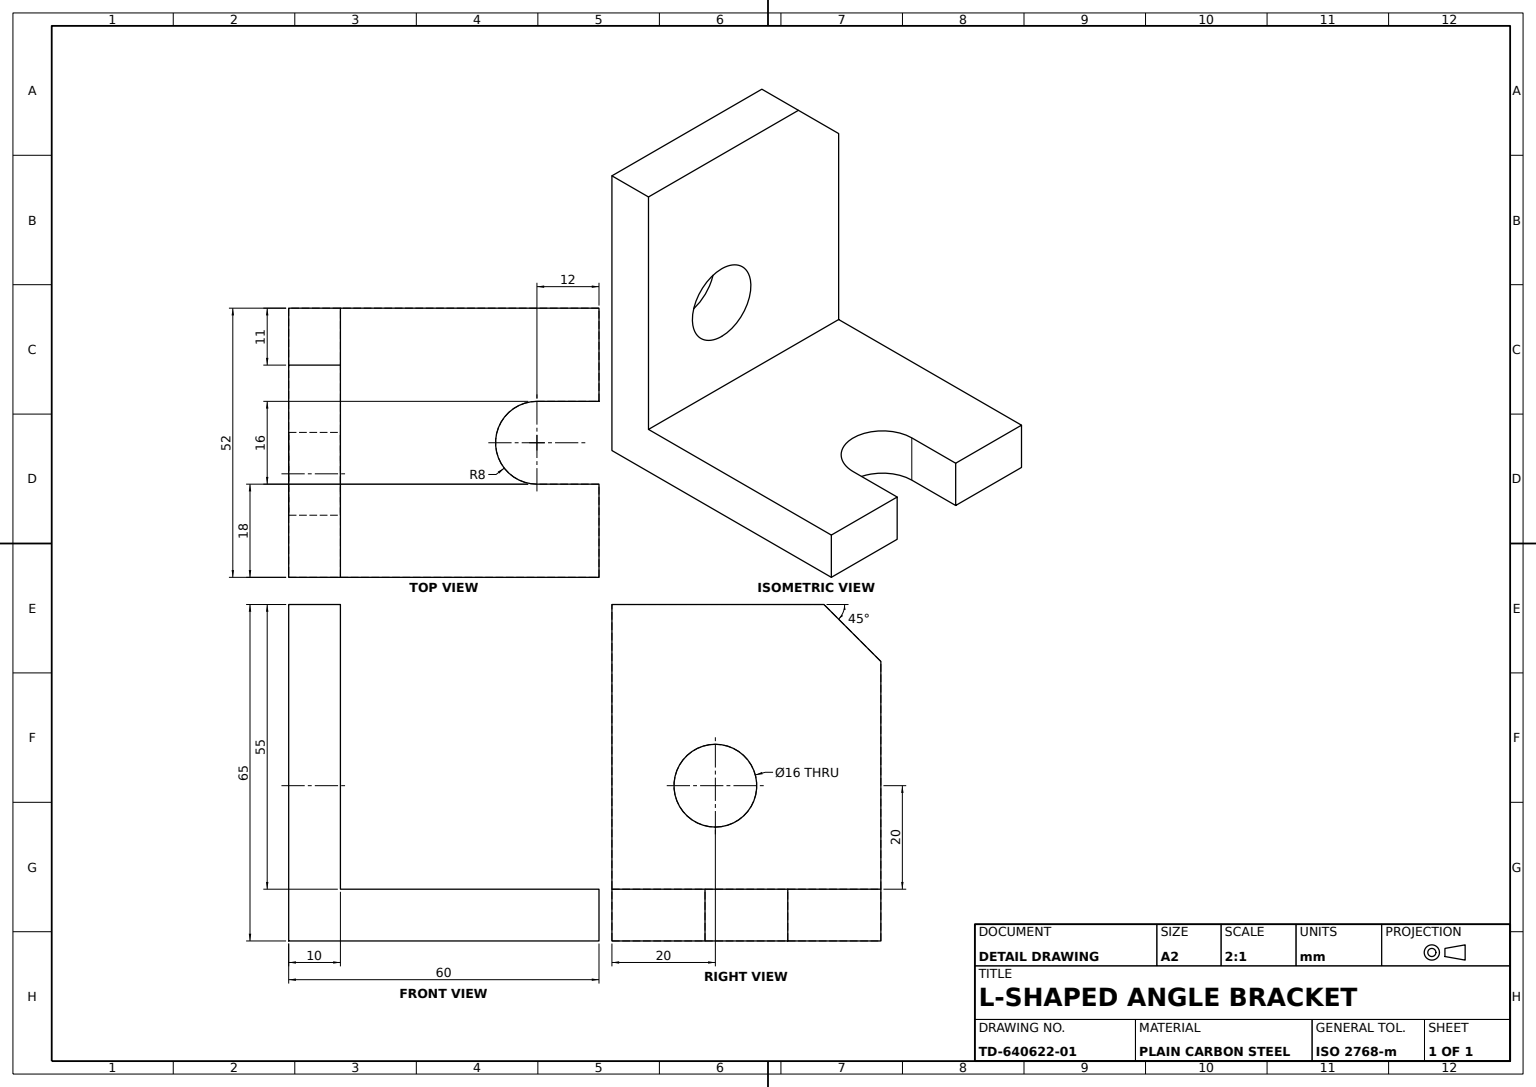
SolidWorks part; units mm, degrees
material "Plain Carbon Steel"
ref_plane "Front Plane" through (0, 0, 0) normal (0, 0, 1) x (1, 0, 0)
ref_plane "Top Plane" through (0, 0, 0) normal (0, 1, 0) x (1, 0, 0)
ref_plane "Right Plane" through (0, 0, 0) normal (1, 0, 0) x (0, 0, -1)
sketch "L-Profile Sketch" plane through (0, 0, 0) normal (0, 0, 1) x (1, 0, 0)
  line L0 (0, 81.9101) -> (0, -77.8652) construction
  line L1 (-117.4157, 0) -> (124.8315, 0) construction
  line L2 (0, 0) -> (0, 65)
  line L3 (0, 65) -> (10, 65)
  line L4 (10, 65) -> (10, 10)
  line L5 (10, 10) -> (60, 10)
  line L6 (60, 10) -> (60, 0)
  line L7 (60, 0) -> (0, 0)
  point P9 (5, 65)
  dimension "D1" = 10
  dimension "D2" = 10
  dimension "D3" = 60
  dimension "D4" = 55
extrude "L-Bracket Body" add sketch "L-Profile Sketch" along normal mid plane 52
sketch "Base Slot Sketch" plane through (0, 10, 0) normal (0, 1, 0) x (1, 0, 0)
  line L0 (-14.5649, 0) -> (74.2265, 0) construction
  line L2 (48, 8) -> (60, 8)
  line L3 (48, -8) -> (60, -8)
  line L5 (60, -26) -> (10, -26) construction
  line L6 (60, -26) -> (60, 26) construction
  line L7 (60, 8) -> (60, -8)
  arc A1 (48, 8) -> (48, -8) centre (48, 0) ccw
  dimension "D1" = 18
  dimension "D2" = 16
  dimension "D3" = 12
extrude "Base U-Slot" cut sketch "Base Slot Sketch" against normal through all contours L2 L7 L3 A1
sketch "Upright Hole Sketch" plane through (10, 0, 0) normal (1, 0, 0) x (0, 0, -1)
  line L0 (-26, 10) -> (-26, 65) construction
  line L1 (-26, 10) -> (-8, 10) construction
  circle A0 centre (-6, 30) radius 8
  dimension "D1" = 16
  dimension "D2" = 20
  dimension "D3" = 20
extrude "Upright Hole Ø16" cut sketch "Upright Hole Sketch" against normal through all
chamfer "Chamfer 11x45°" distance 11 angle 45 1 edges at (5, 65, -26)
